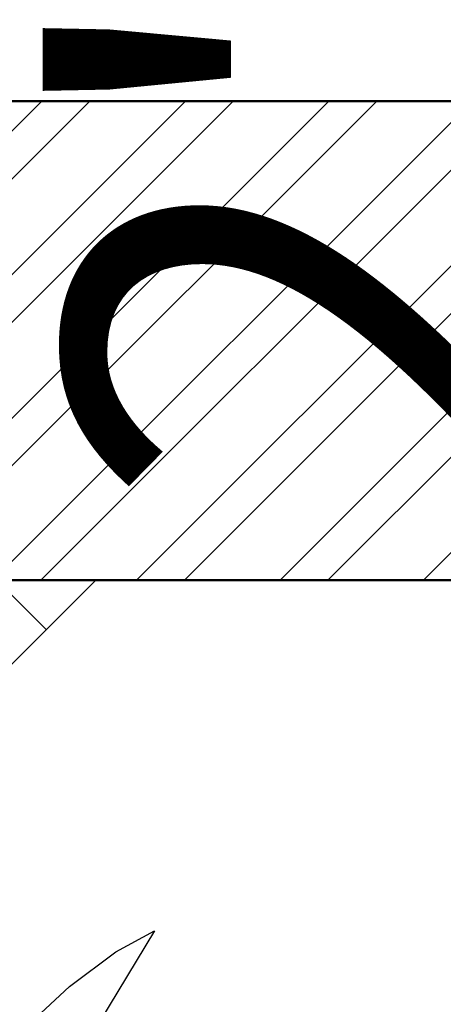
# Model space of a CAD drawing. Units: inches. Extents: x 3590 to 5167, y 65 to 1917.
# Tile 97 of 100: x 5057.33 to 5065.29, y 1789.03 to 1807.53. Entities that reach past the tile are written whole.
import ezdxf

# ---------------------------------------------------------------- set-up
doc = ezdxf.new("R2010")
doc.units = ezdxf.units.IN
for name, color, linetype, lineweight in [('A-ANNO-DIMS', 2, 'Continuous', 18), ('A-FLOR-PATT', 8, 'Continuous', 13), ('A-WALL', 7, 'Continuous', 50), ('A-WALL-PATT', 251, 'Continuous', 13), ('L-PLNT', 94, 'Continuous', 18)]:
    doc.layers.add(name, color=color, linetype=linetype, lineweight=lineweight)
doc.layers.add('DIENHOA', color=3, linetype='Continuous')
doc.styles.get("Standard").update_dxf_attribs({"font": 'arial.ttf'})
doc.dimstyles.new('ISO-25', dxfattribs={"dimtxt": 9, "dimasz": 2.5, "dimexe": 1.25, "dimexo": 0.625, "dimtad": 1, "dimdec": 1, "dimlunit": 3, "dimtxsty": 'Standard', "dimcen": 2.5, "dimadec": 0, "dimazin": 0, "dimtfac": 1, "dimtdec": 1, "dimtmove": 0, "dimatfit": 3, "dimfxl": 1, "dimarcsym": 0})

# ---------------------------------------------------------------- blocks, each defined once
blk = doc.blocks.new('*D101')
at = {"layer": 'A-ANNO-DIMS', "color": 0, "lineweight": -2, "transparency": 16777216}
for p, q in [((4420.274, 1806.624), (4420.274, 1818.615)), ((5080.274, 1806.624), (5080.274, 1818.615)), ((4422.774, 1817.365), (5077.774, 1817.365))]:
    blk.add_line(p, q, dxfattribs=at)
at = {"layer": 'A-ANNO-DIMS', "color": 0, "transparency": 16777216}
for points in [[(4422.774, 1817.781), (4422.774, 1816.948), (4420.274, 1817.365)], [(5077.774, 1817.781), (5077.774, 1816.948), (5080.274, 1817.365)]]:
    blk.add_solid(points, dxfattribs=at)
at = {"layer": 'Defpoints', "color": 0, "transparency": 16777216}
for p in [(5080.274, 1817.365), (4420.274, 1805.999), (5080.274, 1805.999)]:
    blk.add_point(p, dxfattribs=at)
at = {"layer": 'A-ANNO-DIMS', "color": 0, "transparency": 16777216, "insert": (4750.274, 1822.566), "char_height": 9, "attachment_point": 5}
blk.add_mtext("55'", dxfattribs=at)
blk = doc.blocks.new('Cay03_mb')
at = {"layer": 'DIENHOA'}
for points in [[(384.28, 437.45), (342.25, 367.83), (298.14, 301.71), (252.56, 239.37), (206.11, 181.11), (159.39, 127.21), (113.01, 77.96), (67.57, 33.64), (23.69, -5.44)], [(23.69, -5.44), (79.88, 91.71), (134.12, 176.21), (185.81, 248.4), (234.31, 308.65), (279.02, 357.33), (319.33, 394.78), (354.62, 421.37), (384.28, 437.45)]]:
    blk.add_lwpolyline(points, dxfattribs=at)
blk = doc.blocks.new('*D323')
at = {"layer": 'A-ANNO-DIMS', "color": 0, "lineweight": -2, "transparency": 16777216}
for p, q in [((5069.172, 1795.216), (5069.172, 1874.95)), ((5065.437, 1795.216), (5070.422, 1795.216)), ((5069.172, 1769.309), (5069.172, 1792.716)), ((5065.437, 1766.809), (5070.422, 1766.809))]:
    blk.add_line(p, q, dxfattribs=at)
at = {"layer": 'A-ANNO-DIMS', "color": 0, "transparency": 16777216}
for points in [[(5068.756, 1792.716), (5069.589, 1792.716), (5069.172, 1795.216)], [(5068.756, 1769.309), (5069.589, 1769.309), (5069.172, 1766.809)]]:
    blk.add_solid(points, dxfattribs=at)
at = {"layer": 'Defpoints', "color": 0, "transparency": 16777216}
for p in [(5064.812, 1795.216), (5069.172, 1795.216), (5064.812, 1766.809)]:
    blk.add_point(p, dxfattribs=at)
at = {"layer": 'A-ANNO-DIMS', "color": 0, "transparency": 16777216, "insert": (5063.894, 1836.333), "char_height": 9, "attachment_point": 5, "rotation": 90}
blk.add_mtext('2\'-4 1/2" TYP.', dxfattribs=at)

msp = doc.modelspace()

# ---------------------------------------------------------------- hatches: boundary and pattern name
at = {"layer": 'A-FLOR-PATT', "transparency": 33554687}
h = msp.add_hatch(dxfattribs=at)
h.set_pattern_fill('AR-HBONE', color=256, scale=0.2)
h.set_pattern_definition([(45, (-588.972, 0), (0, 28.73682), [60.96, -20.32]), (135, (-574.604, 14.368), (3e-15, 28.73682), [60.96, -20.32])])
h.paths.add_polyline_path([(5071.274, 1796.999), (4933.274, 1796.999), (4933.274, 1753.999), (4962.774, 1753.999, -0.414214), (4928.774, 1719.999), (4933.274, 1718.999), (4933.274, 1334.999), (5071.274, 1334.999)])
h.paths.add_polyline_path([(4951.78, 1521.077), (4951.715, 1521.04), (4951.563, 1520.895)], flags=16)
h.paths.add_polyline_path([(4952.267, 1521.376), (4952.198, 1521.371), (4952.198, 1521.356)], flags=0)
h.paths.add_polyline_path([(4967.051, 1529.728), (4965.231, 1528.694), (4963.411, 1527.714), (4961.756, 1526.851), (4963.589, 1527.449), (4964.036, 1527.478), (4962.975, 1527.249), (4961.76, 1526.852), (4959.792, 1525.834), (4958.005, 1524.895), (4956.24, 1523.93), (4954.504, 1522.919), (4954.129, 1522.682), (4953.361, 1521.997), (4953.366, 1521.998), (4953.605, 1522.064), (4955.106, 1522.761), (4956.921, 1523.434), (4958.678, 1523.915), (4960.358, 1524.2), (4961.945, 1524.286), (4964.171, 1524.108), (4965.958, 1523.309), (4963.863, 1522.976), (4965.187, 1522.499), (4963.366, 1522.497), (4961.545, 1522.487), (4959.764, 1522.461), (4958.304, 1522.419), (4957.974, 1522.388), (4956.307, 1522.232), (4954.718, 1522.071), (4953.251, 1521.899), (4953.525, 1521.623), (4954.331, 1521.379), (4956.243, 1521.23), (4958.039, 1520.93), (4959.684, 1520.483), (4961.16, 1519.896), (4963.107, 1518.8), (4964.393, 1517.325), (4962.973, 1517.726), (4964.558, 1516.661), (4965.407, 1515.708), (4963.507, 1516.322), (4961.68, 1517.005), (4959.935, 1517.745), (4958.282, 1518.528), (4956.732, 1519.343), (4955.295, 1520.175), (4954.672, 1520.572), (4954.513, 1520.627), (4955.658, 1519.318), (4956.703, 1517.982), (4957.644, 1516.647), (4958.485, 1515.334), (4959.55, 1513.524), (4960.438, 1511.769), (4958.841, 1513.62), (4957.452, 1515.325), (4955.819, 1517.459), (4956.665, 1515.448), (4957.111, 1513.923), (4957.447, 1511.714), (4957.076, 1509.793), (4956.538, 1511.11), (4955.992, 1512.569), (4955.444, 1514.125), (4954.898, 1515.735), (4954.357, 1517.356), (4953.824, 1518.943), (4953.305, 1520.452), (4953.065, 1521.116), (4952.971, 1521.146), (4952.949, 1521.086), (4952.73, 1520.199), (4953.37, 1518.024), (4953.757, 1516.373), (4954.051, 1514.765), (4954.264, 1513.221), (4954.471, 1511.131), (4954.497, 1510.402), (4954.409, 1511.76), (4954.264, 1513.221), (4954.051, 1514.765), (4953.757, 1516.373), (4953.37, 1518.024), (4952.877, 1519.698), (4952.716, 1520.141), (4952.533, 1519.059), (4952.374, 1517.789), (4952.219, 1516.312), (4952.046, 1514.6), (4951.833, 1512.626), (4951.557, 1510.363), (4951.203, 1512.168), (4950.852, 1514.339), (4950.985, 1516.376), (4951.66, 1518.286), (4952.593, 1520.481), (4952.357, 1521.13), (4951.855, 1520.328), (4950.839, 1518.908), (4949.777, 1517.587), (4948.916, 1516.617), (4948.111, 1515.256), (4947.089, 1513.554), (4945.889, 1511.615), (4946.326, 1513.402), (4946.562, 1514.249), (4945.528, 1513.327), (4944.581, 1512.531), (4946.018, 1514.508), (4947.204, 1516.048), (4947.893, 1517.313), (4949.307, 1518.764), (4950.414, 1519.767), (4950.451, 1519.806), (4952.267, 1521.376), (4951.645, 1521.493), (4950.404, 1521.18), (4948.044, 1520.359), (4946.119, 1519.452), (4944.572, 1518.475), (4943.35, 1517.443), (4941.997, 1515.92), (4941.661, 1515.275), (4942.813, 1516.99), (4944.572, 1518.475), (4946.119, 1519.452), (4948.044, 1520.359), (4950.404, 1521.18), (4951.645, 1521.493), (4949.647, 1521.868), (4948.6, 1521.756), (4947.126, 1521.57), (4945.42, 1521.348), (4943.45, 1521.105), (4941.183, 1520.856), (4942.86, 1521.613), (4943.873, 1522.03), (4942.952, 1521.909), (4941.41, 1521.485), (4939.543, 1520.67), (4938.968, 1520.226), (4940.733, 1521.299), (4942.952, 1521.909), (4943.702, 1522.008), (4945.894, 1522.7), (4947.565, 1522.714), (4948.921, 1522.566), (4951.131, 1522.183), (4950.971, 1522.297), (4948.129, 1523.006), (4946.035, 1523.707), (4944.232, 1524.521), (4942.707, 1525.461), (4941.444, 1526.537), (4940.43, 1527.761), (4939.649, 1529.143), (4941.421, 1528.122), (4943.147, 1527.132), (4944.841, 1526.175), (4946.514, 1525.25), (4948.179, 1524.359), (4948.365, 1524.263), (4946.475, 1526.045), (4945.181, 1527.54), (4944.19, 1529.033), (4943.496, 1530.54), (4943.278, 1531.36), (4942.498, 1531.919), (4943.114, 1531.762), (4942.959, 1533.659), (4944.14, 1531.989), (4944.612, 1531.323), (4946.202, 1530.463), (4947.486, 1529.509), (4948.79, 1528.226), (4950.368, 1526.237), (4949.485, 1528.155), (4948.851, 1530.123), (4948.491, 1532.041), (4948.381, 1533.918), (4948.501, 1535.76), (4948.827, 1537.573), (4949.418, 1535.565), (4949.957, 1533.569), (4950.464, 1531.586), (4950.961, 1529.617), (4951.391, 1527.954), (4951.724, 1530.687), (4952.201, 1532.58), (4952.889, 1534.33), (4953.77, 1535.951), (4954.827, 1537.46), (4954.521, 1535.39), (4954.273, 1533.937), (4955.58, 1535.663), (4956.748, 1536.739), (4956.159, 1534.78), (4955.589, 1532.873), (4955.043, 1531.006), (4954.525, 1529.166), (4954.038, 1527.341), (4953.638, 1525.733), (4953.611, 1525.586), (4953.398, 1524.166), (4953.382, 1524.009), (4954.07, 1525.476), (4954.912, 1527.022), (4956.136, 1528.894), (4957.847, 1530.577), (4959.376, 1531.54), (4958.256, 1530.104), (4957.143, 1528.663), (4956.066, 1527.243), (4955.056, 1525.871), (4954.141, 1524.571), (4953.352, 1523.372), (4953.311, 1523.303), (4953.273, 1522.925), (4953.261, 1522.382), (4954.103, 1523.373), (4954.63, 1524.284), (4955.961, 1526.358), (4957.23, 1528.13), (4958.421, 1529.609), (4960.037, 1531.368), (4961.374, 1532.375), (4962.101, 1532.77), (4961.07, 1531.061), (4959.987, 1529.438), (4958.869, 1527.908), (4958.15, 1527.007), (4959.803, 1528.003), (4961.589, 1528.793), (4963.391, 1529.328), (4965.211, 1529.632)], flags=16)
h.paths.add_polyline_path([(4962.944, 1523.182), (4961.107, 1523.422), (4960.392, 1523.362), (4962.35, 1523.331)], flags=0)
h.paths.add_polyline_path([(5049.541, 1584.551), (5049.476, 1584.515), (5049.325, 1584.37)], flags=16)
h.paths.add_polyline_path([(5050.028, 1584.851), (5049.959, 1584.845), (5049.959, 1584.83)], flags=0)
h.paths.add_polyline_path([(5042.333, 1581.949), (5043.88, 1582.926), (5045.806, 1583.833), (5048.165, 1584.654), (5049.406, 1584.967), (5047.408, 1585.342), (5046.361, 1585.231), (5044.888, 1585.044), (5043.181, 1584.822), (5041.211, 1584.579), (5038.944, 1584.33), (5040.622, 1585.087), (5041.634, 1585.504), (5040.713, 1585.383), (5039.171, 1584.959), (5037.304, 1584.144), (5036.729, 1583.7), (5038.494, 1584.773), (5040.713, 1585.383), (5041.463, 1585.482), (5043.655, 1586.174), (5045.326, 1586.188), (5046.682, 1586.04), (5048.893, 1585.657), (5048.732, 1585.771), (5045.891, 1586.48), (5043.796, 1587.181), (5041.994, 1587.996), (5040.468, 1588.935), (5039.205, 1590.011), (5038.191, 1591.235), (5037.41, 1592.617), (5039.182, 1591.596), (5040.909, 1590.607), (5042.602, 1589.649), (5044.275, 1588.724), (5045.94, 1587.833), (5046.126, 1587.738), (5044.237, 1589.519), (5042.942, 1591.015), (5041.952, 1592.508), (5041.257, 1594.014), (5041.039, 1594.834), (5040.26, 1595.393), (5040.875, 1595.237), (5040.721, 1597.133), (5041.901, 1595.463), (5042.373, 1594.798), (5043.963, 1593.938), (5045.247, 1592.983), (5046.552, 1591.701), (5048.129, 1589.712), (5047.247, 1591.63), (5046.613, 1593.597), (5046.252, 1595.515), (5046.142, 1597.392), (5046.262, 1599.234), (5046.588, 1601.047), (5047.179, 1599.039), (5047.718, 1597.043), (5048.225, 1595.06), (5048.722, 1593.091), (5049.152, 1591.429), (5049.485, 1594.161), (5049.962, 1596.054), (5050.65, 1597.804), (5051.532, 1599.425), (5052.589, 1600.934), (5052.283, 1598.864), (5052.034, 1597.411), (5053.341, 1599.137), (5054.509, 1600.213), (5053.92, 1598.254), (5053.35, 1596.348), (5052.805, 1594.48), (5052.286, 1592.64), (5051.799, 1590.815), (5051.4, 1589.207), (5051.373, 1589.06), (5051.159, 1587.64), (5051.143, 1587.483), (5051.831, 1588.95), (5052.673, 1590.496), (5053.898, 1592.368), (5055.608, 1594.051), (5057.137, 1595.014), (5056.017, 1593.578), (5054.904, 1592.137), (5053.828, 1590.717), (5052.817, 1589.345), (5051.902, 1588.046), (5051.113, 1586.846), (5051.072, 1586.777), (5051.034, 1586.399), (5051.022, 1585.856), (5051.864, 1586.847), (5052.391, 1587.758), (5053.723, 1589.832), (5054.991, 1591.604), (5056.182, 1593.083), (5057.798, 1594.842), (5059.135, 1595.849), (5059.863, 1596.244), (5058.831, 1594.535), (5057.749, 1592.912), (5056.63, 1591.382), (5055.912, 1590.482), (5057.564, 1591.477), (5059.35, 1592.267), (5061.152, 1592.802), (5062.972, 1593.106), (5064.812, 1593.203), (5062.992, 1592.169), (5061.172, 1591.188), (5059.518, 1590.325), (5061.35, 1590.924), (5061.797, 1590.952), (5060.737, 1590.723), (5059.521, 1590.326), (5057.553, 1589.308), (5055.766, 1588.369), (5054.002, 1587.404), (5052.265, 1586.393), (5051.891, 1586.156), (5051.122, 1585.471), (5051.127, 1585.472), (5051.366, 1585.538), (5052.867, 1586.235), (5054.682, 1586.908), (5056.439, 1587.389), (5058.12, 1587.675), (5059.706, 1587.76), (5061.933, 1587.583), (5063.719, 1586.783), (5061.624, 1586.45), (5062.949, 1585.973), (5061.127, 1585.971), (5059.307, 1585.961), (5057.525, 1585.935), (5056.065, 1585.893), (5055.735, 1585.862), (5054.068, 1585.707), (5052.479, 1585.546), (5051.012, 1585.373), (5051.286, 1585.097), (5052.092, 1584.853), (5054.004, 1584.704), (5055.8, 1584.404), (5057.446, 1583.958), (5058.921, 1583.37), (5060.868, 1582.274), (5062.154, 1580.799), (5060.734, 1581.2), (5062.32, 1580.135), (5063.168, 1579.182), (5061.269, 1579.796), (5059.441, 1580.479), (5057.696, 1581.219), (5056.043, 1582.003), (5054.493, 1582.817), (5053.057, 1583.649), (5052.433, 1584.047), (5052.274, 1584.101), (5053.42, 1582.793), (5054.464, 1581.457), (5055.405, 1580.121), (5056.247, 1578.809), (5057.311, 1576.998), (5058.199, 1575.244), (5056.602, 1577.094), (5055.213, 1578.799), (5053.58, 1580.933), (5054.427, 1578.922), (5054.872, 1577.397), (5055.208, 1575.189), (5054.838, 1573.267), (5054.299, 1574.584), (5053.754, 1576.043), (5053.206, 1577.599), (5052.659, 1579.209), (5052.118, 1580.83), (5051.585, 1582.417), (5051.066, 1583.927), (5050.826, 1584.59), (5050.733, 1584.62), (5050.711, 1584.561), (5050.491, 1583.673), (5051.131, 1581.498), (5051.518, 1579.847), (5051.813, 1578.24), (5052.026, 1576.695), (5052.233, 1574.605), (5052.258, 1573.876), (5052.17, 1575.234), (5052.026, 1576.695), (5051.813, 1578.24), (5051.518, 1579.847), (5051.131, 1581.498), (5050.638, 1583.172), (5050.477, 1583.615), (5050.294, 1582.533), (5050.136, 1581.263), (5049.981, 1579.786), (5049.807, 1578.074), (5049.594, 1576.1), (5049.318, 1573.837), (5048.965, 1575.642), (5048.613, 1577.813), (5048.747, 1579.85), (5049.421, 1581.76), (5050.354, 1583.955), (5050.118, 1584.604), (5049.616, 1583.802), (5048.6, 1582.382), (5047.538, 1581.061), (5046.677, 1580.091), (5045.872, 1578.73), (5044.85, 1577.028), (5043.651, 1575.089), (5044.087, 1576.877), (5044.324, 1577.723), (5043.289, 1576.801), (5042.342, 1576.005), (5043.779, 1577.982), (5044.966, 1579.522), (5045.655, 1580.787), (5047.068, 1582.239), (5048.175, 1583.241), (5048.213, 1583.28), (5050.028, 1584.851), (5049.406, 1584.967), (5048.165, 1584.654), (5045.806, 1583.833), (5043.88, 1582.926), (5042.333, 1581.949), (5041.111, 1580.917), (5039.758, 1579.394), (5039.423, 1578.749), (5040.575, 1580.464)], flags=16)
h.paths.add_polyline_path([(4954.799, 1533.12), (4954.262, 1532.079), (4953.831, 1530.935), (4953.505, 1529.636), (4953.283, 1528.133), (4953.167, 1526.376), (4953.156, 1524.315), (4953.277, 1521.236), (4952.802, 1521.842), (4951.557, 1521.998), (4950.976, 1521.961), (4952.661, 1521.941), (4952.802, 1521.842), (4953.152, 1523.593), (4953.167, 1526.376), (4953.283, 1528.133), (4953.609, 1530.346), (4954.456, 1532.592)], flags=0)
h.paths.add_polyline_path([(5050.563, 1585.316), (5049.318, 1585.472), (5048.737, 1585.435), (5050.422, 1585.415), (5050.563, 1585.316), (5050.914, 1587.067), (5050.928, 1589.851), (5051.045, 1591.607), (5051.371, 1593.82), (5052.217, 1596.066), (5052.56, 1596.594), (5052.024, 1595.554), (5051.592, 1594.409), (5051.266, 1593.11), (5051.045, 1591.607), (5050.928, 1589.851), (5050.918, 1587.789), (5051.038, 1584.71)], flags=0)
h.paths.add_polyline_path([(5058.153, 1586.836), (5060.111, 1586.805), (5060.705, 1586.656), (5058.868, 1586.896)], flags=0)
h.paths.add_polyline_path([(5049.541, 1430.936), (5049.476, 1430.9), (5049.325, 1430.755)], flags=16)
h.paths.add_polyline_path([(5050.028, 1431.236), (5049.959, 1431.231), (5049.959, 1431.215)], flags=0)
h.paths.add_polyline_path([(5046.588, 1447.432), (5047.179, 1445.425), (5047.718, 1443.429), (5048.225, 1441.446), (5048.722, 1439.476), (5049.152, 1437.814), (5049.485, 1440.546), (5049.962, 1442.439), (5050.65, 1444.189), (5051.532, 1445.811), (5052.589, 1447.319), (5052.283, 1445.249), (5052.034, 1443.796), (5053.341, 1445.522), (5054.509, 1446.598), (5053.92, 1444.64), (5053.35, 1442.733), (5052.805, 1440.865), (5052.286, 1439.025), (5051.799, 1437.201), (5051.4, 1435.592), (5051.373, 1435.445), (5051.159, 1434.025), (5051.143, 1433.868), (5051.831, 1435.335), (5052.673, 1436.881), (5053.898, 1438.753), (5055.608, 1440.436), (5057.137, 1441.4), (5056.017, 1439.963), (5054.904, 1438.522), (5053.828, 1437.102), (5052.817, 1435.73), (5051.902, 1434.431), (5051.113, 1433.231), (5051.072, 1433.162), (5051.034, 1432.784), (5051.022, 1432.242), (5051.864, 1433.232), (5052.391, 1434.143), (5053.723, 1436.217), (5054.991, 1437.989), (5056.182, 1439.468), (5057.798, 1441.227), (5059.135, 1442.235), (5059.863, 1442.629), (5058.831, 1440.921), (5057.749, 1439.298), (5056.63, 1437.767), (5055.912, 1436.867), (5057.564, 1437.863), (5059.35, 1438.652), (5061.152, 1439.187), (5062.972, 1439.491), (5064.812, 1439.588), (5062.992, 1438.554), (5061.172, 1437.573), (5059.518, 1436.71), (5061.35, 1437.309), (5061.797, 1437.337), (5060.737, 1437.108), (5059.521, 1436.711), (5057.553, 1435.693), (5055.766, 1434.754), (5054.002, 1433.789), (5052.265, 1432.778), (5051.891, 1432.541), (5051.122, 1431.856), (5051.127, 1431.857), (5051.366, 1431.923), (5052.867, 1432.62), (5054.682, 1433.293), (5056.439, 1433.775), (5058.12, 1434.06), (5059.706, 1434.145), (5061.933, 1433.968), (5063.719, 1433.168), (5061.624, 1432.835), (5062.949, 1432.358), (5061.127, 1432.357), (5059.307, 1432.346), (5057.525, 1432.32), (5056.065, 1432.278), (5055.735, 1432.248), (5054.068, 1432.092), (5052.479, 1431.931), (5051.012, 1431.759), (5051.286, 1431.482), (5052.092, 1431.238), (5054.004, 1431.089), (5055.8, 1430.789), (5057.446, 1430.343), (5058.921, 1429.755), (5060.868, 1428.66), (5062.154, 1427.185), (5060.734, 1427.585), (5062.32, 1426.52), (5063.168, 1425.567), (5061.269, 1426.181), (5059.441, 1426.865), (5057.696, 1427.604), (5056.043, 1428.388), (5054.493, 1429.202), (5053.057, 1430.034), (5052.433, 1430.432), (5052.274, 1430.487), (5053.42, 1429.178), (5054.464, 1427.842), (5055.405, 1426.506), (5056.247, 1425.194), (5057.311, 1423.383), (5058.199, 1421.629), (5056.602, 1423.479), (5055.213, 1425.184), (5053.58, 1427.318), (5054.427, 1425.307), (5054.872, 1423.782), (5055.208, 1421.574), (5054.838, 1419.652), (5054.299, 1420.97), (5053.754, 1422.428), (5053.206, 1423.984), (5052.659, 1425.595), (5052.118, 1427.215), (5051.585, 1428.802), (5051.066, 1430.312), (5050.826, 1430.975), (5050.733, 1431.005), (5050.711, 1430.946), (5050.491, 1430.058), (5051.131, 1427.883), (5051.518, 1426.232), (5051.813, 1424.625), (5052.026, 1423.081), (5052.233, 1420.991), (5052.258, 1420.261), (5052.17, 1421.619), (5052.026, 1423.081), (5051.813, 1424.625), (5051.518, 1426.232), (5051.131, 1427.883), (5050.638, 1429.558), (5050.477, 1430.001), (5050.294, 1428.918), (5050.136, 1427.648), (5049.981, 1426.171), (5049.807, 1424.459), (5049.594, 1422.485), (5049.318, 1420.222), (5048.965, 1422.028), (5048.613, 1424.199), (5048.747, 1426.235), (5049.421, 1428.146), (5050.354, 1430.34), (5050.118, 1430.989), (5049.616, 1430.187), (5048.6, 1428.768), (5047.538, 1427.446), (5046.677, 1426.477), (5045.872, 1425.116), (5044.85, 1423.413), (5043.651, 1421.474), (5044.087, 1423.262), (5044.324, 1424.109), (5043.289, 1423.186), (5042.342, 1422.391), (5043.779, 1424.368), (5044.966, 1425.907), (5045.655, 1427.173), (5047.068, 1428.624), (5048.175, 1429.627), (5048.213, 1429.666), (5050.028, 1431.236), (5049.406, 1431.353), (5048.165, 1431.039), (5045.806, 1430.218), (5043.88, 1429.311), (5042.333, 1428.334), (5041.111, 1427.302), (5039.758, 1425.779), (5039.423, 1425.134), (5040.575, 1426.849), (5042.333, 1428.334), (5043.88, 1429.311), (5045.806, 1430.218), (5048.165, 1431.039), (5049.406, 1431.353), (5047.408, 1431.727), (5046.361, 1431.616), (5044.888, 1431.429), (5043.181, 1431.207), (5041.211, 1430.964), (5038.944, 1430.715), (5040.622, 1431.472), (5041.634, 1431.89), (5040.713, 1431.769), (5039.171, 1431.345), (5037.304, 1430.53), (5036.729, 1430.085), (5038.494, 1431.158), (5040.713, 1431.769), (5041.463, 1431.867), (5043.655, 1432.559), (5045.326, 1432.573), (5046.682, 1432.425), (5048.893, 1432.042), (5048.732, 1432.156), (5045.891, 1432.865), (5043.796, 1433.566), (5041.994, 1434.381), (5040.468, 1435.321), (5039.205, 1436.396), (5038.191, 1437.62), (5037.41, 1439.002), (5039.182, 1437.982), (5040.909, 1436.992), (5042.602, 1436.034), (5044.275, 1435.109), (5045.94, 1434.218), (5046.126, 1434.123), (5044.237, 1435.904), (5042.942, 1437.4), (5041.952, 1438.893), (5041.257, 1440.399), (5041.039, 1441.219), (5040.26, 1441.778), (5040.875, 1441.622), (5040.721, 1443.518), (5041.901, 1441.848), (5042.373, 1441.183), (5043.963, 1440.323), (5045.247, 1439.369), (5046.552, 1438.086), (5048.129, 1436.097), (5047.247, 1438.015), (5046.613, 1439.982), (5046.252, 1441.901), (5046.142, 1443.778), (5046.262, 1445.619)], flags=16)
h.paths.add_polyline_path([(5052.382, 1444.255), (5051.623, 1442.78), (5052.024, 1441.939), (5052.56, 1442.98)], flags=0)
h.paths.add_polyline_path([(5050.563, 1431.701), (5049.318, 1431.857), (5048.737, 1431.821), (5050.422, 1431.8)], flags=0)
h.paths.add_polyline_path([(5058.153, 1433.221), (5060.111, 1433.19), (5060.705, 1433.041), (5058.868, 1433.281)], flags=0)
h.paths.add_polyline_path([(5049.541, 1352.285), (5049.476, 1352.249), (5049.325, 1352.104)], flags=16)
h.paths.add_polyline_path([(5050.028, 1352.585), (5049.959, 1352.58), (5049.959, 1352.564)], flags=0)
h.paths.add_polyline_path([(5046.588, 1368.781), (5047.179, 1366.774), (5047.718, 1364.778), (5048.225, 1362.795), (5048.722, 1360.825), (5049.152, 1359.163), (5049.485, 1361.896), (5049.962, 1363.789), (5050.65, 1365.538), (5051.532, 1367.16), (5052.589, 1368.669), (5052.283, 1366.598), (5052.034, 1365.145), (5053.341, 1366.871), (5054.509, 1367.947), (5053.92, 1365.989), (5053.35, 1364.082), (5052.805, 1362.214), (5052.286, 1360.374), (5051.799, 1358.55), (5051.4, 1356.942), (5051.373, 1356.794), (5051.159, 1355.374), (5051.143, 1355.218), (5051.831, 1356.684), (5052.673, 1358.23), (5053.898, 1360.102), (5055.608, 1361.786), (5057.137, 1362.749), (5056.017, 1361.313), (5054.904, 1359.872), (5053.828, 1358.452), (5052.817, 1357.079), (5051.902, 1355.78), (5051.113, 1354.581), (5051.072, 1354.512), (5051.034, 1354.133), (5051.022, 1353.591), (5051.864, 1354.581), (5052.391, 1355.492), (5053.723, 1357.566), (5054.991, 1359.338), (5056.182, 1360.817), (5057.798, 1362.577), (5059.135, 1363.584), (5059.863, 1363.979), (5058.831, 1362.27), (5057.749, 1360.647), (5056.63, 1359.117), (5055.912, 1358.216), (5057.564, 1359.212), (5059.35, 1360.001), (5061.152, 1360.536), (5062.972, 1360.841), (5064.812, 1360.937), (5062.992, 1359.903), (5061.172, 1358.923), (5059.518, 1358.059), (5061.35, 1358.658), (5061.797, 1358.687), (5060.737, 1358.458), (5059.521, 1358.061), (5057.553, 1357.043), (5055.766, 1356.103), (5054.002, 1355.138), (5052.265, 1354.127), (5051.891, 1353.89), (5051.122, 1353.206), (5051.127, 1353.206), (5051.366, 1353.272), (5052.867, 1353.969), (5054.682, 1354.643), (5056.439, 1355.124), (5058.12, 1355.409), (5059.706, 1355.495), (5061.933, 1355.317), (5063.719, 1354.518), (5061.624, 1354.184), (5062.949, 1353.708), (5061.127, 1353.706), (5059.307, 1353.695), (5057.525, 1353.669), (5056.065, 1353.627), (5055.735, 1353.597), (5054.068, 1353.441), (5052.479, 1353.28), (5051.012, 1353.108), (5051.286, 1352.831), (5052.092, 1352.587), (5054.004, 1352.439), (5055.8, 1352.138), (5057.446, 1351.692), (5058.921, 1351.104), (5060.868, 1350.009), (5062.154, 1348.534), (5060.734, 1348.935), (5062.32, 1347.869), (5063.168, 1346.916), (5061.269, 1347.53), (5059.441, 1348.214), (5057.696, 1348.954), (5056.043, 1349.737), (5054.493, 1350.551), (5053.057, 1351.383), (5052.433, 1351.781), (5052.274, 1351.836), (5053.42, 1350.527), (5054.464, 1349.191), (5055.405, 1347.855), (5056.247, 1346.543), (5057.311, 1344.733), (5058.199, 1342.978), (5056.602, 1344.828), (5055.213, 1346.534), (5053.58, 1348.667), (5054.427, 1346.656), (5054.872, 1345.132), (5055.208, 1342.923), (5054.838, 1341.002), (5054.299, 1342.319), (5053.754, 1343.778), (5053.206, 1345.334), (5052.659, 1346.944), (5052.118, 1348.564), (5051.585, 1350.151), (5051.066, 1351.661), (5050.826, 1352.324), (5050.733, 1352.355), (5050.711, 1352.295), (5050.491, 1351.408), (5051.131, 1349.232), (5051.518, 1347.581), (5051.813, 1345.974), (5052.026, 1344.43), (5052.233, 1342.34), (5052.258, 1341.61), (5052.17, 1342.969), (5052.026, 1344.43), (5051.813, 1345.974), (5051.518, 1347.581), (5051.131, 1349.232), (5050.638, 1350.907), (5050.477, 1351.35), (5050.294, 1350.267), (5050.136, 1348.997), (5049.981, 1347.52), (5049.807, 1345.809), (5049.594, 1343.835), (5049.318, 1341.571), (5048.965, 1343.377), (5048.613, 1345.548), (5048.747, 1347.585), (5049.421, 1349.495), (5050.354, 1351.689), (5050.118, 1352.339), (5049.616, 1351.536), (5048.6, 1350.117), (5047.538, 1348.795), (5046.677, 1347.826), (5045.872, 1346.465), (5044.85, 1344.763), (5043.651, 1342.824), (5044.087, 1344.611), (5044.324, 1345.458), (5043.289, 1344.535), (5042.342, 1343.74), (5043.779, 1345.717), (5044.966, 1347.256), (5045.655, 1348.522), (5047.068, 1349.973), (5048.175, 1350.976), (5048.213, 1351.015), (5050.028, 1352.585), (5049.406, 1352.702), (5048.165, 1352.388), (5045.806, 1351.567), (5043.88, 1350.661), (5042.333, 1349.683), (5041.111, 1348.651), (5039.758, 1347.128), (5039.423, 1346.483), (5040.575, 1348.198), (5042.333, 1349.683), (5043.88, 1350.661), (5045.806, 1351.567), (5048.165, 1352.388), (5049.406, 1352.702), (5047.408, 1353.076), (5046.361, 1352.965), (5044.888, 1352.779), (5043.181, 1352.556), (5041.211, 1352.313), (5038.944, 1352.065), (5040.622, 1352.821), (5041.634, 1353.239), (5040.713, 1353.118), (5039.171, 1352.694), (5037.304, 1351.879), (5036.729, 1351.434), (5038.494, 1352.508), (5040.713, 1353.118), (5041.463, 1353.216), (5043.655, 1353.909), (5045.326, 1353.923), (5046.682, 1353.774), (5048.893, 1353.391), (5048.732, 1353.506), (5045.891, 1354.214), (5043.796, 1354.915), (5041.994, 1355.73), (5040.468, 1356.67), (5039.205, 1357.746), (5038.191, 1358.969), (5037.41, 1360.352), (5039.182, 1359.331), (5040.909, 1358.341), (5042.602, 1357.383), (5044.275, 1356.458), (5045.94, 1355.567), (5046.126, 1355.472), (5044.237, 1357.253), (5042.942, 1358.749), (5041.952, 1360.242), (5041.257, 1361.748), (5041.039, 1362.568), (5040.26, 1363.128), (5040.875, 1362.971), (5040.721, 1364.867), (5041.901, 1363.197), (5042.373, 1362.532), (5043.963, 1361.672), (5045.247, 1360.718), (5046.552, 1359.435), (5048.129, 1357.446), (5047.247, 1359.364), (5046.613, 1361.331), (5046.252, 1363.25), (5046.142, 1365.127), (5046.262, 1366.969)], flags=16)
h.paths.add_polyline_path([(5052.382, 1365.604), (5051.623, 1364.129), (5052.024, 1363.288), (5052.56, 1364.329)], flags=0)
h.paths.add_polyline_path([(4951.78, 1698.041), (4951.715, 1698.005), (4951.563, 1697.859)], flags=16)
h.paths.add_polyline_path([(4952.267, 1698.341), (4952.198, 1698.335), (4952.198, 1698.32)], flags=0)
h.paths.add_polyline_path([(4957.076, 1686.757), (4956.538, 1688.074), (4955.992, 1689.533), (4955.444, 1691.089), (4954.898, 1692.699), (4954.357, 1694.32), (4953.824, 1695.907), (4953.305, 1697.417), (4953.065, 1698.08), (4952.971, 1698.11), (4952.949, 1698.051), (4952.73, 1697.163), (4953.37, 1694.988), (4953.757, 1693.337), (4954.051, 1691.729), (4954.264, 1690.185), (4954.471, 1688.095), (4954.497, 1687.366), (4954.409, 1688.724), (4954.264, 1690.185), (4954.051, 1691.729), (4953.757, 1693.337), (4953.37, 1694.988), (4952.877, 1696.662), (4952.716, 1697.105), (4952.533, 1696.023), (4952.374, 1694.753), (4952.219, 1693.276), (4952.046, 1691.564), (4951.833, 1689.59), (4951.557, 1687.327), (4951.203, 1689.132), (4950.852, 1691.303), (4950.985, 1693.34), (4951.66, 1695.25), (4952.593, 1697.445), (4952.357, 1698.094), (4951.855, 1697.292), (4950.839, 1695.872), (4949.777, 1694.551), (4948.916, 1693.581), (4948.111, 1692.22), (4947.089, 1690.518), (4945.889, 1688.579), (4946.326, 1690.366), (4946.562, 1691.213), (4945.528, 1690.291), (4944.581, 1689.495), (4946.018, 1691.472), (4947.204, 1693.012), (4947.893, 1694.277), (4949.307, 1695.729), (4950.414, 1696.731), (4950.451, 1696.77), (4952.267, 1698.341), (4951.645, 1698.457), (4950.404, 1698.144), (4948.044, 1697.323), (4946.119, 1696.416), (4944.572, 1695.439), (4943.35, 1694.407), (4941.997, 1692.884), (4941.661, 1692.239), (4942.813, 1693.954), (4944.572, 1695.439), (4946.119, 1696.416), (4948.044, 1697.323), (4950.404, 1698.144), (4951.645, 1698.457), (4949.647, 1698.832), (4948.6, 1698.72), (4947.126, 1698.534), (4945.42, 1698.312), (4943.45, 1698.069), (4941.183, 1697.82), (4942.86, 1698.577), (4943.873, 1698.994), (4942.952, 1698.873), (4941.41, 1698.449), (4939.543, 1697.634), (4938.968, 1697.19), (4940.733, 1698.263), (4942.952, 1698.873), (4943.702, 1698.972), (4945.894, 1699.664), (4947.565, 1699.678), (4948.921, 1699.53), (4951.131, 1699.147), (4950.971, 1699.261), (4948.129, 1699.97), (4946.035, 1700.671), (4944.232, 1701.486), (4942.707, 1702.425), (4941.444, 1703.501), (4940.43, 1704.725), (4939.649, 1706.107), (4941.421, 1705.086), (4943.147, 1704.097), (4944.841, 1703.139), (4946.514, 1702.214), (4948.179, 1701.323), (4948.365, 1701.227), (4946.475, 1703.009), (4945.181, 1704.505), (4944.19, 1705.997), (4943.496, 1707.504), (4943.278, 1708.324), (4942.498, 1708.883), (4943.114, 1708.727), (4942.959, 1710.623), (4944.14, 1708.953), (4944.612, 1708.287), (4946.202, 1707.428), (4947.486, 1706.473), (4948.79, 1705.191), (4950.368, 1703.202), (4949.485, 1705.12), (4948.851, 1707.087), (4948.491, 1709.005), (4948.381, 1710.882), (4948.501, 1712.724), (4948.827, 1714.537), (4949.418, 1712.529), (4949.957, 1710.533), (4950.464, 1708.55), (4950.961, 1706.581), (4951.391, 1704.919), (4951.724, 1707.651), (4952.201, 1709.544), (4952.889, 1711.294), (4953.77, 1712.915), (4954.827, 1714.424), (4954.521, 1712.354), (4954.273, 1710.901), (4955.58, 1712.627), (4956.748, 1713.703), (4956.159, 1711.744), (4955.589, 1709.837), (4955.043, 1707.97), (4954.525, 1706.13), (4954.038, 1704.305), (4953.638, 1702.697), (4953.611, 1702.55), (4953.398, 1701.13), (4953.382, 1700.973), (4954.07, 1702.44), (4954.912, 1703.986), (4956.136, 1705.858), (4957.847, 1707.541), (4959.376, 1708.504), (4958.256, 1707.068), (4957.143, 1705.627), (4956.066, 1704.207), (4955.056, 1702.835), (4954.141, 1701.536), (4953.352, 1700.336), (4953.311, 1700.267), (4953.273, 1699.889), (4953.261, 1699.346), (4954.103, 1700.337), (4954.63, 1701.248), (4955.961, 1703.322), (4957.23, 1705.094), (4958.421, 1706.573), (4960.037, 1708.332), (4961.374, 1709.339), (4962.101, 1709.734), (4961.07, 1708.025), (4959.987, 1706.402), (4958.869, 1704.872), (4958.15, 1703.972), (4959.803, 1704.967), (4961.589, 1705.757), (4963.391, 1706.292), (4965.211, 1706.596), (4967.051, 1706.692), (4965.231, 1705.659), (4963.411, 1704.678), (4961.756, 1703.815), (4963.589, 1704.413), (4964.036, 1704.442), (4962.975, 1704.213), (4961.76, 1703.816), (4959.792, 1702.798), (4958.005, 1701.859), (4956.24, 1700.894), (4954.504, 1699.883), (4954.129, 1699.646), (4953.361, 1698.961), (4953.366, 1698.962), (4953.605, 1699.028), (4955.106, 1699.725), (4956.921, 1700.398), (4958.678, 1700.879), (4960.358, 1701.164), (4961.945, 1701.25), (4964.171, 1701.073), (4965.958, 1700.273), (4963.863, 1699.94), (4965.187, 1699.463), (4963.366, 1699.461), (4961.545, 1699.451), (4959.764, 1699.425), (4958.304, 1699.383), (4957.974, 1699.352), (4956.307, 1699.197), (4954.718, 1699.036), (4953.251, 1698.863), (4953.525, 1698.587), (4954.331, 1698.343), (4956.243, 1698.194), (4958.039, 1697.894), (4959.684, 1697.447), (4961.16, 1696.86), (4963.107, 1695.764), (4964.393, 1694.289), (4962.973, 1694.69), (4964.558, 1693.625), (4965.407, 1692.672), (4963.507, 1693.286), (4961.68, 1693.969), (4959.935, 1694.709), (4958.282, 1695.492), (4956.732, 1696.307), (4955.295, 1697.139), (4954.672, 1697.536), (4954.513, 1697.591), (4955.658, 1696.282), (4956.703, 1694.946), (4957.644, 1693.611), (4958.485, 1692.298), (4959.55, 1690.488), (4960.438, 1688.733), (4958.841, 1690.584), (4957.452, 1692.289), (4955.819, 1694.423), (4956.665, 1692.412), (4957.111, 1690.887), (4957.447, 1688.678)], flags=16)
h.paths.add_polyline_path([(5050.563, 1353.05), (5049.318, 1353.207), (5048.737, 1353.17), (5050.422, 1353.15)], flags=0)
h.paths.add_polyline_path([(4951.78, 1351.486), (4951.715, 1351.45), (4951.563, 1351.305)], flags=16)
h.paths.add_polyline_path([(4952.267, 1351.786), (4952.198, 1351.78), (4952.198, 1351.765)], flags=0)
h.paths.add_polyline_path([(4954.827, 1367.869), (4954.521, 1365.799), (4954.273, 1364.346), (4955.58, 1366.072), (4956.748, 1367.148), (4956.159, 1365.19), (4955.589, 1363.283), (4955.043, 1361.415), (4954.525, 1359.575), (4954.038, 1357.751), (4953.638, 1356.142), (4953.611, 1355.995), (4953.398, 1354.575), (4953.382, 1354.418), (4954.07, 1355.885), (4954.912, 1357.431), (4956.136, 1359.303), (4957.847, 1360.986), (4959.376, 1361.95), (4958.256, 1360.513), (4957.143, 1359.072), (4956.066, 1357.652), (4955.056, 1356.28), (4954.141, 1354.981), (4953.352, 1353.781), (4953.311, 1353.712), (4953.273, 1353.334), (4953.261, 1352.792), (4954.103, 1353.782), (4954.63, 1354.693), (4955.961, 1356.767), (4957.23, 1358.539), (4958.421, 1360.018), (4960.037, 1361.777), (4961.374, 1362.785), (4962.101, 1363.179), (4961.07, 1361.471), (4959.987, 1359.848), (4958.869, 1358.317), (4958.15, 1357.417), (4959.803, 1358.413), (4961.589, 1359.202), (4963.391, 1359.737), (4965.211, 1360.041), (4967.051, 1360.138), (4965.231, 1359.104), (4963.411, 1358.123), (4961.756, 1357.26), (4963.589, 1357.859), (4964.036, 1357.887), (4962.975, 1357.658), (4961.76, 1357.261), (4959.792, 1356.243), (4958.005, 1355.304), (4956.24, 1354.339), (4954.504, 1353.328), (4954.129, 1353.091), (4953.361, 1352.406), (4953.366, 1352.407), (4953.605, 1352.473), (4955.106, 1353.17), (4956.921, 1353.843), (4958.678, 1354.325), (4960.358, 1354.61), (4961.945, 1354.695), (4964.171, 1354.518), (4965.958, 1353.718), (4963.863, 1353.385), (4965.187, 1352.908), (4963.366, 1352.907), (4961.545, 1352.896), (4959.764, 1352.87), (4958.304, 1352.828), (4957.974, 1352.798), (4956.307, 1352.642), (4954.718, 1352.481), (4953.251, 1352.309), (4953.525, 1352.032), (4954.331, 1351.788), (4956.243, 1351.639), (4958.039, 1351.339), (4959.684, 1350.893), (4961.16, 1350.305), (4963.107, 1349.21), (4964.393, 1347.735), (4962.973, 1348.135), (4964.558, 1347.07), (4965.407, 1346.117), (4963.507, 1346.731), (4961.68, 1347.414), (4959.935, 1348.154), (4958.282, 1348.938), (4956.732, 1349.752), (4955.295, 1350.584), (4954.672, 1350.982), (4954.513, 1351.036), (4955.658, 1349.728), (4956.703, 1348.392), (4957.644, 1347.056), (4958.485, 1345.744), (4959.55, 1343.933), (4960.438, 1342.179), (4958.841, 1344.029), (4957.452, 1345.734), (4955.819, 1347.868), (4956.665, 1345.857), (4957.111, 1344.332), (4957.447, 1342.124), (4957.076, 1340.202), (4956.538, 1341.52), (4955.992, 1342.978), (4955.444, 1344.534), (4954.898, 1346.145), (4954.357, 1347.765), (4953.824, 1349.352), (4953.305, 1350.862), (4953.065, 1351.525), (4952.971, 1351.555), (4952.949, 1351.496), (4952.73, 1350.608), (4953.37, 1348.433), (4953.757, 1346.782), (4954.051, 1345.175), (4954.264, 1343.631), (4954.471, 1341.541), (4954.497, 1340.811), (4954.409, 1342.169), (4954.264, 1343.631), (4954.051, 1345.175), (4953.757, 1346.782), (4953.37, 1348.433), (4952.877, 1350.108), (4952.716, 1350.551), (4952.533, 1349.468), (4952.374, 1348.198), (4952.219, 1346.721), (4952.046, 1345.009), (4951.833, 1343.035), (4951.557, 1340.772), (4951.203, 1342.578), (4950.852, 1344.749), (4950.985, 1346.785), (4951.66, 1348.696), (4952.593, 1350.89), (4952.357, 1351.539), (4951.855, 1350.737), (4950.839, 1349.318), (4949.777, 1347.996), (4948.916, 1347.027), (4948.111, 1345.665), (4947.089, 1343.963), (4945.889, 1342.024), (4946.326, 1343.812), (4946.562, 1344.659), (4945.528, 1343.736), (4944.581, 1342.941), (4946.018, 1344.918), (4947.204, 1346.457), (4947.893, 1347.723), (4949.307, 1349.174), (4950.414, 1350.177), (4950.451, 1350.216), (4952.267, 1351.786), (4951.645, 1351.903), (4950.404, 1351.589), (4948.044, 1350.768), (4946.119, 1349.861), (4944.572, 1348.884), (4943.35, 1347.852), (4941.997, 1346.329), (4941.661, 1345.684), (4942.813, 1347.399), (4944.572, 1348.884), (4946.119, 1349.861), (4948.044, 1350.768), (4950.404, 1351.589), (4951.645, 1351.903), (4949.647, 1352.277), (4948.6, 1352.166), (4947.126, 1351.979), (4945.42, 1351.757), (4943.45, 1351.514), (4941.183, 1351.265), (4942.86, 1352.022), (4943.873, 1352.44), (4942.952, 1352.319), (4941.41, 1351.895), (4939.543, 1351.08), (4938.968, 1350.635), (4940.733, 1351.708), (4942.952, 1352.319), (4943.702, 1352.417), (4945.894, 1353.109), (4947.565, 1353.123), (4948.921, 1352.975), (4951.131, 1352.592), (4950.971, 1352.706), (4948.129, 1353.415), (4946.035, 1354.116), (4944.232, 1354.931), (4942.707, 1355.871), (4941.444, 1356.946), (4940.43, 1358.17), (4939.649, 1359.552), (4941.421, 1358.532), (4943.147, 1357.542), (4944.841, 1356.584), (4946.514, 1355.659), (4948.179, 1354.768), (4948.365, 1354.673), (4946.475, 1356.454), (4945.181, 1357.95), (4944.19, 1359.443), (4943.496, 1360.949), (4943.278, 1361.769), (4942.498, 1362.328), (4943.114, 1362.172), (4942.959, 1364.068), (4944.14, 1362.398), (4944.612, 1361.733), (4946.202, 1360.873), (4947.486, 1359.919), (4948.79, 1358.636), (4950.368, 1356.647), (4949.485, 1358.565), (4948.851, 1360.532), (4948.491, 1362.451), (4948.381, 1364.328), (4948.501, 1366.169), (4948.827, 1367.982), (4949.418, 1365.975), (4949.957, 1363.979), (4950.464, 1361.995), (4950.961, 1360.026), (4951.391, 1358.364), (4951.724, 1361.096), (4952.201, 1362.989), (4952.889, 1364.739), (4953.77, 1366.361)], flags=16)
h.paths.add_polyline_path([(4954.799, 1363.53), (4954.262, 1362.489), (4953.831, 1361.344), (4953.505, 1360.045), (4953.283, 1358.543), (4953.167, 1356.786), (4953.156, 1354.724), (4953.277, 1351.646), (4952.802, 1352.251), (4951.557, 1352.407), (4950.976, 1352.371), (4952.661, 1352.35), (4952.802, 1352.251), (4953.152, 1354.002), (4953.167, 1356.786), (4953.283, 1358.543), (4953.609, 1360.755), (4954.456, 1363.001)], flags=0)
h.paths.add_polyline_path([(4952.802, 1698.806), (4951.557, 1698.962), (4950.976, 1698.925), (4952.661, 1698.905), (4952.802, 1698.806), (4953.152, 1700.557), (4953.167, 1703.34), (4953.283, 1705.097), (4953.609, 1707.31), (4954.456, 1709.556), (4954.799, 1710.084), (4954.262, 1709.043), (4953.831, 1707.899), (4953.505, 1706.6), (4953.283, 1705.097), (4953.167, 1703.34), (4953.156, 1701.279), (4953.277, 1698.2)], flags=0)
h.paths.add_polyline_path([(4962.944, 1700.146), (4961.107, 1700.386), (4960.392, 1700.326), (4962.35, 1700.295)], flags=0)
h.paths.add_polyline_path([(5058.153, 1354.57), (5060.111, 1354.539), (5060.705, 1354.391), (5058.868, 1354.631)], flags=0)
h.paths.add_polyline_path([(4962.944, 1353.591), (4961.107, 1353.831), (4960.392, 1353.771), (4962.35, 1353.74)], flags=0)
h.paths.add_polyline_path([(5049.541, 1778.72), (5049.476, 1778.684), (5049.325, 1778.539)], flags=16)
h.paths.add_polyline_path([(5050.028, 1779.02), (5049.959, 1779.014), (5049.959, 1778.999)], flags=0)
h.paths.add_polyline_path([(5052.258, 1768.045), (5052.17, 1769.403), (5052.026, 1770.864), (5051.813, 1772.409), (5051.518, 1774.016), (5051.131, 1775.667), (5050.638, 1777.341), (5050.477, 1777.784), (5050.294, 1776.702), (5050.136, 1775.432), (5049.981, 1773.955), (5049.807, 1772.243), (5049.594, 1770.269), (5049.318, 1768.006), (5048.965, 1769.811), (5048.613, 1771.982), (5048.747, 1774.019), (5049.421, 1775.929), (5050.354, 1778.124), (5050.118, 1778.773), (5049.616, 1777.971), (5048.6, 1776.551), (5047.538, 1775.23), (5046.677, 1774.26), (5045.872, 1772.899), (5044.85, 1771.197), (5043.651, 1769.258), (5044.087, 1771.046), (5044.324, 1771.892), (5043.289, 1770.97), (5042.342, 1770.174), (5043.779, 1772.151), (5044.966, 1773.691), (5045.655, 1774.956), (5047.068, 1776.408), (5048.175, 1777.41), (5048.213, 1777.449), (5050.028, 1779.02), (5049.406, 1779.136), (5048.165, 1778.823), (5045.806, 1778.002), (5043.88, 1777.095), (5042.333, 1776.118), (5041.111, 1775.086), (5039.758, 1773.563), (5039.423, 1772.918), (5040.575, 1774.633), (5042.333, 1776.118), (5043.88, 1777.095), (5045.806, 1778.002), (5048.165, 1778.823), (5049.406, 1779.136), (5047.408, 1779.511), (5046.361, 1779.4), (5044.888, 1779.213), (5043.181, 1778.991), (5041.211, 1778.748), (5038.944, 1778.499), (5040.622, 1779.256), (5041.634, 1779.673), (5040.713, 1779.552), (5039.171, 1779.128), (5037.304, 1778.313), (5036.729, 1777.869), (5038.494, 1778.942), (5040.713, 1779.552), (5041.463, 1779.651), (5043.655, 1780.343), (5045.326, 1780.357), (5046.682, 1780.209), (5048.893, 1779.826), (5048.732, 1779.94), (5045.891, 1780.649), (5043.796, 1781.35), (5041.994, 1782.165), (5040.468, 1783.104), (5039.205, 1784.18), (5038.191, 1785.404), (5037.41, 1786.786), (5039.182, 1785.765), (5040.909, 1784.776), (5042.602, 1783.818), (5044.275, 1782.893), (5045.94, 1782.002), (5046.126, 1781.907), (5044.237, 1783.688), (5042.942, 1785.184), (5041.952, 1786.677), (5041.257, 1788.183), (5041.039, 1789.003), (5040.26, 1789.562), (5040.875, 1789.406), (5040.721, 1791.302), (5041.901, 1789.632), (5042.373, 1788.967), (5043.963, 1788.107), (5045.247, 1787.152), (5046.552, 1785.87), (5048.129, 1783.881), (5047.247, 1785.799), (5046.613, 1787.766), (5046.252, 1789.684), (5046.142, 1791.561), (5046.262, 1793.403), (5046.588, 1795.216), (5047.179, 1793.208), (5047.718, 1791.213), (5048.225, 1789.229), (5048.722, 1787.26), (5049.152, 1785.598), (5049.485, 1788.33), (5049.962, 1790.223), (5050.65, 1791.973), (5051.532, 1793.594), (5052.589, 1795.103), (5052.283, 1793.033), (5052.034, 1791.58), (5053.341, 1793.306), (5054.509, 1794.382), (5053.92, 1792.423), (5053.35, 1790.517), (5052.805, 1788.649), (5052.286, 1786.809), (5051.799, 1784.984), (5051.4, 1783.376), (5051.373, 1783.229), (5051.159, 1781.809), (5051.143, 1781.652), (5051.831, 1783.119), (5052.673, 1784.665), (5053.898, 1786.537), (5055.608, 1788.22), (5057.137, 1789.183), (5056.017, 1787.747), (5054.904, 1786.306), (5053.828, 1784.886), (5052.817, 1783.514), (5051.902, 1782.215), (5051.113, 1781.015), (5051.072, 1780.946), (5051.034, 1780.568), (5051.022, 1780.025), (5051.864, 1781.016), (5052.391, 1781.927), (5053.723, 1784.001), (5054.991, 1785.773), (5056.182, 1787.252), (5057.798, 1789.011), (5059.135, 1790.018), (5059.863, 1790.413), (5058.831, 1788.704), (5057.749, 1787.081), (5056.63, 1785.551), (5055.912, 1784.651), (5057.564, 1785.646), (5059.35, 1786.436), (5061.152, 1786.971), (5062.972, 1787.275), (5064.812, 1787.372), (5062.992, 1786.338), (5061.172, 1785.357), (5059.518, 1784.494), (5061.35, 1785.093), (5061.797, 1785.121), (5060.737, 1784.892), (5059.521, 1784.495), (5057.553, 1783.477), (5055.766, 1782.538), (5054.002, 1781.573), (5052.265, 1780.562), (5051.891, 1780.325), (5051.122, 1779.64), (5051.127, 1779.641), (5051.366, 1779.707), (5052.867, 1780.404), (5054.682, 1781.077), (5056.439, 1781.558), (5058.12, 1781.844), (5059.706, 1781.929), (5061.933, 1781.752), (5063.719, 1780.952), (5061.624, 1780.619), (5062.949, 1780.142), (5061.127, 1780.14), (5059.307, 1780.13), (5057.525, 1780.104), (5056.065, 1780.062), (5055.735, 1780.031), (5054.068, 1779.876), (5052.479, 1779.715), (5051.012, 1779.542), (5051.286, 1779.266), (5052.092, 1779.022), (5054.004, 1778.873), (5055.8, 1778.573), (5057.446, 1778.127), (5058.921, 1777.539), (5060.868, 1776.443), (5062.154, 1774.968), (5060.734, 1775.369), (5062.32, 1774.304), (5063.168, 1773.351), (5061.269, 1773.965), (5059.441, 1774.648), (5057.696, 1775.388), (5056.043, 1776.172), (5054.493, 1776.986), (5053.057, 1777.818), (5052.433, 1778.216), (5052.274, 1778.27), (5053.42, 1776.962), (5054.464, 1775.626), (5055.405, 1774.29), (5056.247, 1772.978), (5057.311, 1771.167), (5058.199, 1769.413), (5056.602, 1771.263), (5055.213, 1772.968), (5053.58, 1775.102), (5054.427, 1773.091), (5054.872, 1771.566), (5055.208, 1769.358), (5054.838, 1767.436), (5054.299, 1768.753), (5053.754, 1770.212), (5053.206, 1771.768), (5052.659, 1773.378), (5052.118, 1774.999), (5051.585, 1776.586), (5051.066, 1778.096), (5050.826, 1778.759), (5050.733, 1778.789), (5050.711, 1778.73), (5050.491, 1777.842), (5051.131, 1775.667), (5051.518, 1774.016), (5051.813, 1772.409), (5052.026, 1770.864), (5052.233, 1768.774)], flags=16)
h.paths.add_polyline_path([(5050.563, 1779.485), (5049.318, 1779.641), (5048.737, 1779.604), (5050.422, 1779.584), (5050.563, 1779.485), (5050.914, 1781.236), (5050.928, 1784.02), (5051.045, 1785.776), (5051.371, 1787.989), (5052.217, 1790.235), (5052.56, 1790.763), (5052.024, 1789.723), (5051.592, 1788.578), (5051.266, 1787.279), (5051.045, 1785.776), (5050.928, 1784.02), (5050.918, 1781.958), (5051.038, 1778.879)], flags=0)
h.paths.add_polyline_path([(5058.153, 1781.005), (5060.111, 1780.974), (5060.705, 1780.825), (5058.868, 1781.065)], flags=0)
at = {"layer": 'A-WALL-PATT', "transparency": 33554687}
h = msp.add_hatch(dxfattribs=at)
h.set_pattern_fill('ANSI32', color=256, scale=0.2)
h.paths.add_polyline_path([(4684.274, 1805.999), (4591.274, 1805.999), (4591.274, 1796.999), (4639.274, 1796.999), (4639.274, 1790.999), (4648.274, 1790.999), (4648.274, 1796.999), (4684.274, 1796.999)])
h.paths.add_polyline_path([(4543.274, 1805.999), (4420.274, 1805.999), (4420.274, 1784.999), (4429.274, 1784.999), (4429.274, 1796.999), (4445.919, 1796.999), (4543.274, 1796.999)])
h.paths.add_polyline_path([(4828.274, 1805.999), (4744.274, 1805.999), (4744.274, 1796.999), (4828.274, 1796.999)])
h.paths.add_polyline_path([(4648.274, 1754.999), (4639.274, 1754.999), (4639.274, 1655.999), (4546.274, 1655.999), (4546.274, 1649.999), (4549.274, 1649.999), (4549.274, 1553.999), (4429.274, 1553.999), (4429.274, 1583.999), (4420.274, 1583.999), (4420.274, 1538.999), (4429.274, 1538.999), (4429.274, 1544.999), (4639.274, 1544.999), (4639.274, 1538.999), (4648.274, 1538.999), (4648.274, 1559.999), (4639.274, 1559.999), (4639.274, 1553.999), (4555.274, 1553.999), (4555.274, 1649.999), (4639.274, 1649.999), (4639.274, 1589.999), (4648.274, 1589.999)])
h.paths.add_polyline_path([(4516.274, 1655.999), (4429.274, 1655.999), (4429.274, 1736.999), (4420.274, 1736.999), (4420.274, 1619.999), (4429.274, 1619.999), (4429.274, 1649.999), (4516.274, 1649.999)], flags=17)
h.paths.add_polyline_path([(5080.274, 1805.999), (4888.274, 1805.999), (4888.274, 1796.999), (4924.274, 1796.999), (4924.274, 1754.999), (4933.274, 1754.999), (4933.274, 1796.999), (5071.274, 1796.999), (5071.274, 1334.999), (4933.274, 1334.999), (4933.274, 1565.999), (4924.274, 1565.999), (4924.274, 1334.999), (4898.774, 1334.999), (4898.774, 1325.999), (5080.274, 1325.999)])
h.paths.add_polyline_path([(4933.274, 1718.999), (4924.274, 1718.999), (4924.274, 1637.999), (4933.274, 1637.999)], flags=17)
h.paths.add_polyline_path([(4802.774, 1334.999), (4777.274, 1334.999), (4777.274, 1502.999), (4756.274, 1502.999), (4756.274, 1493.999), (4768.274, 1493.999), (4768.274, 1430.999), (4696.274, 1430.999), (4696.274, 1493.999), (4708.274, 1493.999), (4708.274, 1502.999), (4639.274, 1502.999), (4639.274, 1493.999), (4687.274, 1493.999), (4687.274, 1430.999), (4681.274, 1430.999), (4681.274, 1421.999), (4768.274, 1421.999), (4768.274, 1334.999), (4726.274, 1334.999), (4726.274, 1325.999), (4802.774, 1325.999)])
h.paths.add_polyline_path([(4690.274, 1334.999), (4648.274, 1334.999), (4648.274, 1352.867), (4648.274, 1421.999), (4651.274, 1421.999), (4651.274, 1430.999), (4639.274, 1430.999), (4639.274, 1334.999), (4633.274, 1334.999), (4633.274, 1325.999), (4690.274, 1325.999)])
h.paths.add_polyline_path([(4585.274, 1334.999), (4584.724, 1334.999), (4429.274, 1334.999), (4429.274, 1490.999), (4420.274, 1490.999), (4420.274, 1325.999), (4585.274, 1325.999)])

# ---------------------------------------------------------------- linework, layer by layer
at = {"layer": 'A-WALL'}
msp.add_line((4933.274, 1796.999), (5071.274, 1796.999), dxfattribs=at)
msp.add_lwpolyline([(5080.274, 1805.999), (5080.274, 1325.999), (4420.274, 1325.999), (4420.274, 1805.999)], close=True, dxfattribs=at)

# ---------------------------------------------------------------- block references
at = {"layer": 'L-PLNT', "xscale": 0.0245452446402784, "yscale": 0.0245452446402784, "zscale": 0.0245452446402784}
msp.add_blockref('Cay03_mb', (5050.431, 1779.676), dxfattribs=at)

# ---------------------------------------------------------------- dimensions: what is measured, and where the dimension line sits
at = {"layer": 'A-ANNO-DIMS'}
dim = msp.add_linear_dim(base=(5069.172, 1795.216), p1=(5064.812, 1766.809), p2=(5064.812, 1795.216), angle=90, text='<> TYP.', dimstyle='ISO-25', override={"dimdec": 1, "dimlfac": 1, "dimrnd": 0, "dimzin": 1, "dimdsep": 46, "dimlunit": 4, "dimfrac": 2}, dxfattribs=at)
dim.commit()
dim.dimension.update_dxf_attribs({"geometry": '*D323', "text_midpoint": (5063.894, 1836.333)})
dim = msp.add_linear_dim(base=(5080.274, 1817.365), p1=(4420.274, 1805.999), p2=(5080.274, 1805.999), dimstyle='ISO-25', override={"dimclrd": 0, "dimclre": 0, "dimclrt": 0}, dxfattribs=at)
dim.commit()
dim.dimension.update_dxf_attribs({"geometry": '*D101', "text_midpoint": (4750.274, 1822.566)})

doc.saveas('drawing.dxf')
